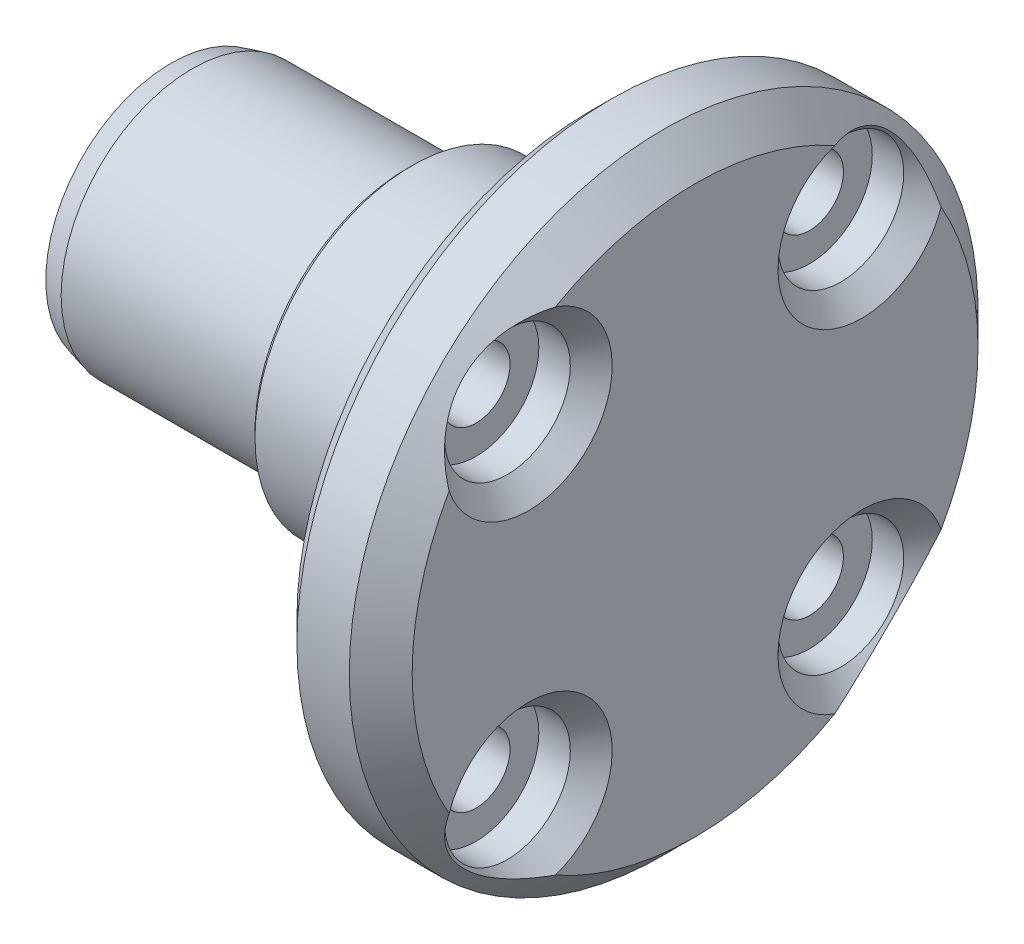
ISO-10303-21;
HEADER;
FILE_DESCRIPTION(('STEP AP214'),'2;1');
FILE_NAME('part.step','',(''),(''),'','','');
FILE_SCHEMA(('AUTOMOTIVE_DESIGN { 1 0 10303 214 1 1 1 1 }'));
ENDSEC;
DATA;
#1=APPLICATION_CONTEXT('core data for automotive mechanical design processes');
#2=APPLICATION_PROTOCOL_DEFINITION('international standard','automotive_design',2000,#1);
#3=PRODUCT_CONTEXT('',#1,'mechanical');
#4=PRODUCT('Part','Part','',(#3));
#5=PRODUCT_RELATED_PRODUCT_CATEGORY('part','',(#4));
#6=PRODUCT_DEFINITION_FORMATION('','',#4);
#7=PRODUCT_DEFINITION_CONTEXT('part definition',#1,'design');
#8=PRODUCT_DEFINITION('design','',#6,#7);
#9=PRODUCT_DEFINITION_SHAPE('','',#8);
#10=(LENGTH_UNIT() NAMED_UNIT(*) SI_UNIT(.MILLI.,.METRE.));
#11=(NAMED_UNIT(*) PLANE_ANGLE_UNIT() SI_UNIT($,.RADIAN.));
#12=(NAMED_UNIT(*) SI_UNIT($,.STERADIAN.) SOLID_ANGLE_UNIT());
#13=UNCERTAINTY_MEASURE_WITH_UNIT(LENGTH_MEASURE(1.E-05),#10,'distance_accuracy_value','');
#14=(GEOMETRIC_REPRESENTATION_CONTEXT(3) GLOBAL_UNCERTAINTY_ASSIGNED_CONTEXT((#13)) GLOBAL_UNIT_ASSIGNED_CONTEXT((#10,
#11,#12)) REPRESENTATION_CONTEXT('',''));
#15=CARTESIAN_POINT('',(0.,0.,0.));
#16=DIRECTION('',(0.,0.,1.));
#17=DIRECTION('',(1.,0.,0.));
#18=AXIS2_PLACEMENT_3D('',#15,#16,#17);
#19=CARTESIAN_POINT('',(0.,15.9099025766973,-15.9099025766973));
#20=DIRECTION('',(1.,0.,0.));
#21=DIRECTION('',(0.,0.,-1.));
#22=AXIS2_PLACEMENT_3D('',#19,#20,#21);
#23=CYLINDRICAL_SURFACE('',#22,3.25);
#24=CARTESIAN_POINT('',(40.,15.9099025766973,-15.9099025766973));
#25=DIRECTION('',(1.,0.,0.));
#26=DIRECTION('',(0.,0.,-1.));
#27=AXIS2_PLACEMENT_3D('',#24,#25,#26);
#28=CIRCLE('',#27,3.25);
#29=CARTESIAN_POINT('',(40.,15.9099025766973,-19.1599025766973));
#30=VERTEX_POINT('',#29);
#31=EDGE_CURVE('E154',#30,#30,#28,.T.);
#32=ORIENTED_EDGE('',*,*,#31,.F.);
#33=EDGE_LOOP('',(#32));
#34=FACE_BOUND('',#33,.T.);
#35=CARTESIAN_POINT('',(45.,15.9099025766973,-15.9099025766973));
#36=DIRECTION('',(1.,0.,0.));
#37=DIRECTION('',(0.,0.,-1.));
#38=AXIS2_PLACEMENT_3D('',#35,#36,#37);
#39=CIRCLE('',#38,3.25);
#40=CARTESIAN_POINT('',(45.,15.9099025766973,-19.1599025766973));
#41=VERTEX_POINT('',#40);
#42=EDGE_CURVE('E146',#41,#41,#39,.F.);
#43=ORIENTED_EDGE('',*,*,#42,.F.);
#44=EDGE_LOOP('',(#43));
#45=FACE_BOUND('',#44,.T.);
#46=ADVANCED_FACE('F43',(#34,#45),#23,.F.);
#47=CARTESIAN_POINT('',(0.,-15.9099025766973,-15.9099025766973));
#48=DIRECTION('',(1.,0.,0.));
#49=DIRECTION('',(0.,0.,-1.));
#50=AXIS2_PLACEMENT_3D('',#47,#48,#49);
#51=CYLINDRICAL_SURFACE('',#50,3.25);
#52=CARTESIAN_POINT('',(40.,-15.9099025766973,-15.9099025766973));
#53=DIRECTION('',(1.,0.,0.));
#54=DIRECTION('',(0.,0.,-1.));
#55=AXIS2_PLACEMENT_3D('',#52,#53,#54);
#56=CIRCLE('',#55,3.25);
#57=CARTESIAN_POINT('',(40.,-15.9099025766973,-19.1599025766973));
#58=VERTEX_POINT('',#57);
#59=EDGE_CURVE('E326',#58,#58,#56,.T.);
#60=ORIENTED_EDGE('',*,*,#59,.F.);
#61=EDGE_LOOP('',(#60));
#62=FACE_BOUND('',#61,.T.);
#63=CARTESIAN_POINT('',(45.,-15.9099025766973,-15.9099025766973));
#64=DIRECTION('',(1.,0.,0.));
#65=DIRECTION('',(0.,0.,-1.));
#66=AXIS2_PLACEMENT_3D('',#63,#64,#65);
#67=CIRCLE('',#66,3.25);
#68=CARTESIAN_POINT('',(45.,-15.9099025766973,-19.1599025766973));
#69=VERTEX_POINT('',#68);
#70=EDGE_CURVE('E147',#69,#69,#67,.F.);
#71=ORIENTED_EDGE('',*,*,#70,.F.);
#72=EDGE_LOOP('',(#71));
#73=FACE_BOUND('',#72,.T.);
#74=ADVANCED_FACE('F217',(#62,#73),#51,.F.);
#75=CARTESIAN_POINT('',(0.,-15.9099025766972,15.9099025766974));
#76=DIRECTION('',(1.,0.,0.));
#77=DIRECTION('',(0.,0.,-1.));
#78=AXIS2_PLACEMENT_3D('',#75,#76,#77);
#79=CYLINDRICAL_SURFACE('',#78,3.25);
#80=CARTESIAN_POINT('',(40.,-15.9099025766972,15.9099025766974));
#81=DIRECTION('',(1.,0.,0.));
#82=DIRECTION('',(0.,0.,-1.));
#83=AXIS2_PLACEMENT_3D('',#80,#81,#82);
#84=CIRCLE('',#83,3.25);
#85=CARTESIAN_POINT('',(40.,-15.9099025766972,12.6599025766974));
#86=VERTEX_POINT('',#85);
#87=EDGE_CURVE('E332',#86,#86,#84,.T.);
#88=ORIENTED_EDGE('',*,*,#87,.F.);
#89=EDGE_LOOP('',(#88));
#90=FACE_BOUND('',#89,.T.);
#91=CARTESIAN_POINT('',(45.,-15.9099025766972,15.9099025766974));
#92=DIRECTION('',(1.,0.,0.));
#93=DIRECTION('',(0.,0.,-1.));
#94=AXIS2_PLACEMENT_3D('',#91,#92,#93);
#95=CIRCLE('',#94,3.25);
#96=CARTESIAN_POINT('',(45.,-15.9099025766972,12.6599025766974));
#97=VERTEX_POINT('',#96);
#98=EDGE_CURVE('E145',#97,#97,#95,.F.);
#99=ORIENTED_EDGE('',*,*,#98,.F.);
#100=EDGE_LOOP('',(#99));
#101=FACE_BOUND('',#100,.T.);
#102=ADVANCED_FACE('F224',(#90,#101),#79,.F.);
#103=CARTESIAN_POINT('',(0.,15.9099025766975,15.9099025766972));
#104=DIRECTION('',(1.,0.,0.));
#105=DIRECTION('',(0.,0.,-1.));
#106=AXIS2_PLACEMENT_3D('',#103,#104,#105);
#107=CYLINDRICAL_SURFACE('',#106,3.25);
#108=CARTESIAN_POINT('',(40.,15.9099025766975,15.9099025766972));
#109=DIRECTION('',(1.,0.,0.));
#110=DIRECTION('',(0.,0.,-1.));
#111=AXIS2_PLACEMENT_3D('',#108,#109,#110);
#112=CIRCLE('',#111,3.25);
#113=CARTESIAN_POINT('',(40.,15.9099025766975,12.6599025766972));
#114=VERTEX_POINT('',#113);
#115=EDGE_CURVE('E337',#114,#114,#112,.T.);
#116=ORIENTED_EDGE('',*,*,#115,.F.);
#117=EDGE_LOOP('',(#116));
#118=FACE_BOUND('',#117,.T.);
#119=CARTESIAN_POINT('',(45.,15.9099025766975,15.9099025766972));
#120=DIRECTION('',(1.,0.,0.));
#121=DIRECTION('',(0.,0.,-1.));
#122=AXIS2_PLACEMENT_3D('',#119,#120,#121);
#123=CIRCLE('',#122,3.25);
#124=CARTESIAN_POINT('',(45.,15.9099025766975,12.6599025766972));
#125=VERTEX_POINT('',#124);
#126=EDGE_CURVE('E138',#125,#125,#123,.F.);
#127=ORIENTED_EDGE('',*,*,#126,.F.);
#128=EDGE_LOOP('',(#127));
#129=FACE_BOUND('',#128,.T.);
#130=ADVANCED_FACE('F235',(#118,#129),#107,.F.);
#131=CARTESIAN_POINT('',(0.,0.,0.));
#132=DIRECTION('',(1.,0.,0.));
#133=DIRECTION('',(0.,0.,-1.));
#134=AXIS2_PLACEMENT_3D('',#131,#132,#133);
#135=PLANE('',#134);
#136=CARTESIAN_POINT('',(0.,0.,0.));
#137=DIRECTION('',(1.,0.,0.));
#138=DIRECTION('',(0.,0.,-1.));
#139=AXIS2_PLACEMENT_3D('',#136,#137,#138);
#140=CIRCLE('',#139,11.9641016151378);
#141=CARTESIAN_POINT('',(0.,0.,-11.9641016151378));
#142=VERTEX_POINT('',#141);
#143=EDGE_CURVE('E287',#142,#142,#140,.F.);
#144=ORIENTED_EDGE('',*,*,#143,.T.);
#145=EDGE_LOOP('',(#144));
#146=FACE_BOUND('',#145,.T.);
#147=ADVANCED_FACE('F253',(#146),#135,.F.);
#148=CARTESIAN_POINT('',(-413.520497285991,0.,0.));
#149=DIRECTION('',(-1.,0.,0.));
#150=DIRECTION('',(0.,0.,1.));
#151=AXIS2_PLACEMENT_3D('',#148,#149,#150);
#152=CYLINDRICAL_SURFACE('',#151,12.5);
#153=CARTESIAN_POINT('',(21.5,0.,0.));
#154=DIRECTION('',(1.,0.,0.));
#155=DIRECTION('',(0.,0.,-1.));
#156=AXIS2_PLACEMENT_3D('',#153,#154,#155);
#157=CIRCLE('',#156,12.5);
#158=CARTESIAN_POINT('',(21.5,0.,-12.5));
#159=VERTEX_POINT('',#158);
#160=EDGE_CURVE('E134',#159,#159,#157,.F.);
#161=ORIENTED_EDGE('',*,*,#160,.T.);
#162=EDGE_LOOP('',(#161));
#163=FACE_BOUND('',#162,.T.);
#164=CARTESIAN_POINT('',(1.99999999999984,0.,0.));
#165=DIRECTION('',(1.,0.,0.));
#166=DIRECTION('',(0.,0.,-1.));
#167=AXIS2_PLACEMENT_3D('',#164,#165,#166);
#168=CIRCLE('',#167,12.5);
#169=CARTESIAN_POINT('',(1.99999999999984,0.,-12.5));
#170=VERTEX_POINT('',#169);
#171=EDGE_CURVE('E282',#170,#170,#168,.T.);
#172=ORIENTED_EDGE('',*,*,#171,.T.);
#173=EDGE_LOOP('',(#172));
#174=FACE_BOUND('',#173,.T.);
#175=ADVANCED_FACE('F252',(#163,#174),#152,.T.);
#176=CARTESIAN_POINT('',(22.5,12.5,0.));
#177=DIRECTION('',(1.,0.,0.));
#178=DIRECTION('',(0.,0.,-1.));
#179=AXIS2_PLACEMENT_3D('',#176,#177,#178);
#180=PLANE('',#179);
#181=CARTESIAN_POINT('',(22.5,0.,0.));
#182=DIRECTION('',(1.,0.,0.));
#183=DIRECTION('',(0.,0.,-1.));
#184=AXIS2_PLACEMENT_3D('',#181,#182,#183);
#185=CIRCLE('',#184,13.5);
#186=CARTESIAN_POINT('',(22.5,0.,-13.5));
#187=VERTEX_POINT('',#186);
#188=EDGE_CURVE('E131',#187,#187,#185,.T.);
#189=ORIENTED_EDGE('',*,*,#188,.T.);
#190=EDGE_LOOP('',(#189));
#191=FACE_BOUND('',#190,.T.);
#192=CARTESIAN_POINT('',(22.5,0.,0.));
#193=DIRECTION('',(1.,0.,0.));
#194=DIRECTION('',(0.,0.,-1.));
#195=AXIS2_PLACEMENT_3D('',#192,#193,#194);
#196=CIRCLE('',#195,14.5);
#197=CARTESIAN_POINT('',(22.5,0.,-14.5));
#198=VERTEX_POINT('',#197);
#199=EDGE_CURVE('E283',#198,#198,#196,.F.);
#200=ORIENTED_EDGE('',*,*,#199,.T.);
#201=EDGE_LOOP('',(#200));
#202=FACE_BOUND('',#201,.T.);
#203=ADVANCED_FACE('F250',(#191,#202),#180,.F.);
#204=CARTESIAN_POINT('',(-413.520497285991,0.,0.));
#205=DIRECTION('',(-1.,0.,0.));
#206=DIRECTION('',(0.,0.,1.));
#207=AXIS2_PLACEMENT_3D('',#204,#205,#206);
#208=CYLINDRICAL_SURFACE('',#207,15.);
#209=CARTESIAN_POINT('',(39.,0.,0.));
#210=DIRECTION('',(1.,0.,0.));
#211=DIRECTION('',(0.,0.,-1.));
#212=AXIS2_PLACEMENT_3D('',#209,#210,#211);
#213=CIRCLE('',#212,15.);
#214=CARTESIAN_POINT('',(39.,0.,-15.));
#215=VERTEX_POINT('',#214);
#216=EDGE_CURVE('E119',#215,#215,#213,.F.);
#217=ORIENTED_EDGE('',*,*,#216,.T.);
#218=EDGE_LOOP('',(#217));
#219=FACE_BOUND('',#218,.T.);
#220=CARTESIAN_POINT('',(23.,0.,0.));
#221=DIRECTION('',(1.,0.,0.));
#222=DIRECTION('',(0.,0.,-1.));
#223=AXIS2_PLACEMENT_3D('',#220,#221,#222);
#224=CIRCLE('',#223,15.);
#225=CARTESIAN_POINT('',(23.,0.,-15.));
#226=VERTEX_POINT('',#225);
#227=EDGE_CURVE('E279',#226,#226,#224,.T.);
#228=ORIENTED_EDGE('',*,*,#227,.T.);
#229=EDGE_LOOP('',(#228));
#230=FACE_BOUND('',#229,.T.);
#231=ADVANCED_FACE('F243',(#219,#230),#208,.T.);
#232=CARTESIAN_POINT('',(40.,15.,0.));
#233=DIRECTION('',(1.,0.,0.));
#234=DIRECTION('',(0.,0.,-1.));
#235=AXIS2_PLACEMENT_3D('',#232,#233,#234);
#236=PLANE('',#235);
#237=ORIENTED_EDGE('',*,*,#115,.T.);
#238=EDGE_LOOP('',(#237));
#239=FACE_BOUND('',#238,.T.);
#240=ORIENTED_EDGE('',*,*,#87,.T.);
#241=EDGE_LOOP('',(#240));
#242=FACE_BOUND('',#241,.T.);
#243=ORIENTED_EDGE('',*,*,#59,.T.);
#244=EDGE_LOOP('',(#243));
#245=FACE_BOUND('',#244,.T.);
#246=ORIENTED_EDGE('',*,*,#31,.T.);
#247=EDGE_LOOP('',(#246));
#248=FACE_BOUND('',#247,.T.);
#249=CARTESIAN_POINT('',(40.,0.,0.));
#250=DIRECTION('',(1.,0.,0.));
#251=DIRECTION('',(0.,0.,-1.));
#252=AXIS2_PLACEMENT_3D('',#249,#250,#251);
#253=CIRCLE('',#252,16.);
#254=CARTESIAN_POINT('',(40.,0.,-16.));
#255=VERTEX_POINT('',#254);
#256=EDGE_CURVE('E126',#255,#255,#253,.T.);
#257=ORIENTED_EDGE('',*,*,#256,.T.);
#258=EDGE_LOOP('',(#257));
#259=FACE_BOUND('',#258,.T.);
#260=CARTESIAN_POINT('',(40.,0.,0.));
#261=DIRECTION('',(1.,0.,0.));
#262=DIRECTION('',(0.,0.,-1.));
#263=AXIS2_PLACEMENT_3D('',#260,#261,#262);
#264=CIRCLE('',#263,28.);
#265=CARTESIAN_POINT('',(40.,0.,-28.));
#266=VERTEX_POINT('',#265);
#267=EDGE_CURVE('E281',#266,#266,#264,.F.);
#268=ORIENTED_EDGE('',*,*,#267,.T.);
#269=EDGE_LOOP('',(#268));
#270=FACE_BOUND('',#269,.T.);
#271=ADVANCED_FACE('F239',(#239,#242,#245,#248,#259,#270),#236,.F.);
#272=CARTESIAN_POINT('',(-413.520497285991,0.,0.));
#273=DIRECTION('',(-1.,0.,0.));
#274=DIRECTION('',(0.,0.,1.));
#275=AXIS2_PLACEMENT_3D('',#272,#273,#274);
#276=CYLINDRICAL_SURFACE('',#275,30.);
#277=CARTESIAN_POINT('',(47.,0.,0.));
#278=DIRECTION('',(-1.,0.,0.));
#279=DIRECTION('',(0.,0.,1.));
#280=AXIS2_PLACEMENT_3D('',#277,#278,#279);
#281=CIRCLE('',#280,30.);
#282=CARTESIAN_POINT('',(47.,0.,30.));
#283=VERTEX_POINT('',#282);
#284=EDGE_CURVE('E123',#283,#283,#281,.T.);
#285=ORIENTED_EDGE('',*,*,#284,.T.);
#286=EDGE_LOOP('',(#285));
#287=FACE_BOUND('',#286,.T.);
#288=CARTESIAN_POINT('',(42.,0.,0.));
#289=DIRECTION('',(1.,0.,0.));
#290=DIRECTION('',(0.,0.,-1.));
#291=AXIS2_PLACEMENT_3D('',#288,#289,#290);
#292=CIRCLE('',#291,30.);
#293=CARTESIAN_POINT('',(42.,0.,-30.));
#294=VERTEX_POINT('',#293);
#295=EDGE_CURVE('E291',#294,#294,#292,.T.);
#296=ORIENTED_EDGE('',*,*,#295,.T.);
#297=EDGE_LOOP('',(#296));
#298=FACE_BOUND('',#297,.T.);
#299=ADVANCED_FACE('F240',(#287,#298),#276,.T.);
#300=CARTESIAN_POINT('',(50.,30.,0.));
#301=DIRECTION('',(-1.,0.,0.));
#302=DIRECTION('',(0.,0.,1.));
#303=AXIS2_PLACEMENT_3D('',#300,#301,#302);
#304=PLANE('',#303);
#305=CARTESIAN_POINT('',(50.,0.,0.));
#306=DIRECTION('',(-1.,0.,0.));
#307=DIRECTION('',(0.,0.,1.));
#308=AXIS2_PLACEMENT_3D('',#305,#306,#307);
#309=CIRCLE('',#308,26.9999999999999);
#310=CARTESIAN_POINT('',(50.,13.3272740892091,23.4815622425573));
#311=VERTEX_POINT('',#310);
#312=CARTESIAN_POINT('',(50.,-13.3272740892072,23.4815622425584));
#313=VERTEX_POINT('',#312);
#314=EDGE_CURVE('E122',#311,#313,#309,.F.);
#315=ORIENTED_EDGE('',*,*,#314,.T.);
#316=CARTESIAN_POINT('',(50.,-15.9099025766972,15.9099025766975));
#317=DIRECTION('',(-1.,0.,0.));
#318=DIRECTION('',(0.,0.,1.));
#319=AXIS2_PLACEMENT_3D('',#316,#317,#318);
#320=CIRCLE('',#319,8.00000000000129);
#321=CARTESIAN_POINT('',(50.,-23.4815622425582,13.3272740892076));
#322=VERTEX_POINT('',#321);
#323=EDGE_CURVE('E157',#313,#322,#320,.T.);
#324=ORIENTED_EDGE('',*,*,#323,.T.);
#325=CARTESIAN_POINT('',(50.,-23.4815622425586,-13.3272740892067));
#326=VERTEX_POINT('',#325);
#327=EDGE_CURVE('E111',#322,#326,#309,.F.);
#328=ORIENTED_EDGE('',*,*,#327,.T.);
#329=CARTESIAN_POINT('',(50.,-15.9099025766975,-15.9099025766972));
#330=DIRECTION('',(-1.,0.,0.));
#331=DIRECTION('',(0.,0.,1.));
#332=AXIS2_PLACEMENT_3D('',#329,#330,#331);
#333=CIRCLE('',#332,8.00000000000167);
#334=CARTESIAN_POINT('',(50.,-13.3272740892071,-23.4815622425584));
#335=VERTEX_POINT('',#334);
#336=EDGE_CURVE('E94',#326,#335,#333,.T.);
#337=ORIENTED_EDGE('',*,*,#336,.T.);
#338=CARTESIAN_POINT('',(50.,13.3272740892082,-23.4815622425578));
#339=VERTEX_POINT('',#338);
#340=EDGE_CURVE('E108',#335,#339,#309,.F.);
#341=ORIENTED_EDGE('',*,*,#340,.T.);
#342=CARTESIAN_POINT('',(50.,15.9099025766972,-15.9099025766974));
#343=DIRECTION('',(-1.,0.,0.));
#344=DIRECTION('',(0.,0.,1.));
#345=AXIS2_PLACEMENT_3D('',#342,#343,#344);
#346=CIRCLE('',#345,8.00000000000041);
#347=CARTESIAN_POINT('',(50.,23.4815622425576,-13.3272740892086));
#348=VERTEX_POINT('',#347);
#349=EDGE_CURVE('E113',#339,#348,#346,.T.);
#350=ORIENTED_EDGE('',*,*,#349,.T.);
#351=CARTESIAN_POINT('',(50.,23.4815622425576,13.3272740892087));
#352=VERTEX_POINT('',#351);
#353=EDGE_CURVE('E117',#348,#352,#309,.F.);
#354=ORIENTED_EDGE('',*,*,#353,.T.);
#355=CARTESIAN_POINT('',(50.,15.9099025766975,15.9099025766972));
#356=DIRECTION('',(-1.,0.,0.));
#357=DIRECTION('',(0.,0.,1.));
#358=AXIS2_PLACEMENT_3D('',#355,#356,#357);
#359=CIRCLE('',#358,8.00000000000001);
#360=EDGE_CURVE('E115',#352,#311,#359,.T.);
#361=ORIENTED_EDGE('',*,*,#360,.T.);
#362=EDGE_LOOP('',(#315,#324,#328,#337,#341,#350,#354,#361));
#363=FACE_BOUND('',#362,.T.);
#364=ADVANCED_FACE('F106',(#363),#304,.F.);
#365=CARTESIAN_POINT('',(0.,0.,0.));
#366=DIRECTION('',(1.,0.,0.));
#367=DIRECTION('',(0.,0.,-1.));
#368=AXIS2_PLACEMENT_3D('',#365,#366,#367);
#369=CONICAL_SURFACE('',#368,11.9641016151378,0.261799387799145);
#370=ORIENTED_EDGE('',*,*,#171,.F.);
#371=EDGE_LOOP('',(#370));
#372=FACE_BOUND('',#371,.T.);
#373=ORIENTED_EDGE('',*,*,#143,.F.);
#374=EDGE_LOOP('',(#373));
#375=FACE_BOUND('',#374,.T.);
#376=ADVANCED_FACE('F236',(#372,#375),#369,.T.);
#377=CARTESIAN_POINT('',(22.5,0.,0.));
#378=DIRECTION('',(1.,0.,0.));
#379=DIRECTION('',(0.,0.,-1.));
#380=AXIS2_PLACEMENT_3D('',#377,#378,#379);
#381=CONICAL_SURFACE('',#380,14.5,0.785398163397459);
#382=ORIENTED_EDGE('',*,*,#227,.F.);
#383=EDGE_LOOP('',(#382));
#384=FACE_BOUND('',#383,.T.);
#385=ORIENTED_EDGE('',*,*,#199,.F.);
#386=EDGE_LOOP('',(#385));
#387=FACE_BOUND('',#386,.T.);
#388=ADVANCED_FACE('F261',(#384,#387),#381,.T.);
#389=CARTESIAN_POINT('',(40.,0.,0.));
#390=DIRECTION('',(1.,0.,0.));
#391=DIRECTION('',(0.,0.,-1.));
#392=AXIS2_PLACEMENT_3D('',#389,#390,#391);
#393=CONICAL_SURFACE('',#392,28.,0.785398163397449);
#394=ORIENTED_EDGE('',*,*,#295,.F.);
#395=EDGE_LOOP('',(#394));
#396=FACE_BOUND('',#395,.T.);
#397=ORIENTED_EDGE('',*,*,#267,.F.);
#398=EDGE_LOOP('',(#397));
#399=FACE_BOUND('',#398,.T.);
#400=ADVANCED_FACE('F179',(#396,#399),#393,.T.);
#401=CARTESIAN_POINT('',(47.,0.,0.));
#402=DIRECTION('',(-1.,0.,0.));
#403=DIRECTION('',(0.,0.,1.));
#404=AXIS2_PLACEMENT_3D('',#401,#402,#403);
#405=CONICAL_SURFACE('',#404,30.,0.785398163397453);
#406=ORIENTED_EDGE('',*,*,#327,.F.);
#407=CARTESIAN_POINT('',(50.,-23.4815622425582,13.3272740892076));
#408=CARTESIAN_POINT('',(49.8623244860714,-23.4501261029835,13.6615809085384));
#409=CARTESIAN_POINT('',(49.729847524722,-23.4060193855582,13.9971220723128));
#410=CARTESIAN_POINT('',(49.4770962688516,-23.2901308846266,14.6690349677443));
#411=CARTESIAN_POINT('',(49.3568557273336,-23.2182750397604,15.005406507941));
#412=CARTESIAN_POINT('',(49.130364607533,-23.044098697827,15.6778378924903));
#413=CARTESIAN_POINT('',(49.0242166728757,-22.9415706847337,16.0138794484197));
#414=CARTESIAN_POINT('',(48.8295157157687,-22.7044055048471,16.6793648815442));
#415=CARTESIAN_POINT('',(48.7409419766265,-22.569806560804,17.0088161103876));
#416=CARTESIAN_POINT('',(48.6077926268345,-22.3134344018236,17.5581018946699));
#417=CARTESIAN_POINT('',(48.5580366664604,-22.2002670031255,17.7807268217913));
#418=CARTESIAN_POINT('',(48.4690049388357,-21.9577334422976,18.2191201908146));
#419=CARTESIAN_POINT('',(48.4297264752503,-21.8283714603836,18.4348903841346));
#420=CARTESIAN_POINT('',(48.3624731952472,-21.5541150927226,18.857096419529));
#421=CARTESIAN_POINT('',(48.3344595512093,-21.409276276618,19.0635621083674));
#422=CARTESIAN_POINT('',(48.2900903846549,-21.1042659036492,19.4661796679442));
#423=CARTESIAN_POINT('',(48.2737347141895,-20.9440945413963,19.6623316695422));
#424=CARTESIAN_POINT('',(48.2529782152301,-20.6086471955302,20.0434409834205));
#425=CARTESIAN_POINT('',(48.2486285347439,-20.4333098597996,20.2283471279417));
#426=CARTESIAN_POINT('',(48.2521243327868,-20.0694228288624,20.5845437957797));
#427=CARTESIAN_POINT('',(48.2599699356902,-19.8808729989263,20.7558341802167));
#428=CARTESIAN_POINT('',(48.287695077658,-19.492041858547,21.0836731200354));
#429=CARTESIAN_POINT('',(48.307580891907,-19.2917544798609,21.2402139389581));
#430=CARTESIAN_POINT('',(48.3589796658958,-18.8812901088742,21.5376067757385));
#431=CARTESIAN_POINT('',(48.3904925605129,-18.6711131719704,21.6784588814622));
#432=CARTESIAN_POINT('',(48.4632222571038,-18.2502598824055,21.9393150015014));
#433=CARTESIAN_POINT('',(48.5040565993866,-18.0398638868651,22.0598800270941));
#434=CARTESIAN_POINT('',(48.5952975981466,-17.6131386639482,22.2858852932756));
#435=CARTESIAN_POINT('',(48.6457040569396,-17.3968095591817,22.3913258461373));
#436=CARTESIAN_POINT('',(48.7554740246399,-16.9591702576477,22.5874835389128));
#437=CARTESIAN_POINT('',(48.8148583395111,-16.7378495339623,22.6781654349596));
#438=CARTESIAN_POINT('',(48.9417252990491,-16.2920222701561,22.8448996268596));
#439=CARTESIAN_POINT('',(49.009209793041,-16.067515012884,22.9209485715568));
#440=CARTESIAN_POINT('',(49.1870466711792,-15.5038602181733,23.0933821941168));
#441=CARTESIAN_POINT('',(49.3019800268374,-15.1634383076975,23.1809636218455));
#442=CARTESIAN_POINT('',(49.5458457510178,-14.4814174201221,23.3265072868126));
#443=CARTESIAN_POINT('',(49.6747791170565,-14.1398183608304,23.3844674118187));
#444=CARTESIAN_POINT('',(49.9435868289789,-13.4601137155175,23.4728252608893));
#445=CARTESIAN_POINT('',(50.0833809907119,-13.1220001534713,23.5034073571108));
#446=CARTESIAN_POINT('',(50.3002689328816,-12.6175056752025,23.5307727053113));
#447=CARTESIAN_POINT('',(50.3736805300881,-12.4499677956794,23.5368133104263));
#448=CARTESIAN_POINT('',(50.5227811371483,-12.1157505422478,23.543025962824));
#449=CARTESIAN_POINT('',(50.5984706720326,-11.9490713767898,23.5431966466475));
#450=CARTESIAN_POINT('',(50.6752004593743,-11.7829063540803,23.5405647490687));
#451=B_SPLINE_CURVE_WITH_KNOTS('',3,(#407,#408,#409,#410,#411,#412,#413,#414,#415,#416,#417,
#418,#419,#420,#421,#422,#423,#424,#425,#426,#427,#428,#429,#430,#431,#432,#433,#434,#435,#436,
#437,#438,#439,#440,#441,#442,#443,#444,#445,#446,#447,#448,#449,#450),.UNSPECIFIED.,.F.,.F.,(4,
2,2,2,2,2,2,2,2,2,2,2,2,2,2,2,2,2,2,2,2,4),(0.,1.08886818828556,2.1806628363172,
3.28001794745952,4.37806932271815,5.14126897214217,5.90427202580824,6.66462213880451,
7.42496260218441,8.18853731054611,8.95211980631814,9.71610061326384,10.4800771412568,
11.2170440676808,11.953995775853,12.6926823009605,13.4315377950644,14.5392751691669,
15.6470915226554,16.7473901203332,17.296345280672,17.8454279508924),.UNSPECIFIED.);
#452=EDGE_CURVE('E187',#322,#313,#451,.T.);
#453=ORIENTED_EDGE('',*,*,#452,.T.);
#454=ORIENTED_EDGE('',*,*,#314,.F.);
#455=CARTESIAN_POINT('',(50.,13.3272740892091,23.4815622425573));
#456=CARTESIAN_POINT('',(49.8623244860714,13.6615809085398,23.4501261029826));
#457=CARTESIAN_POINT('',(49.729847524722,13.9971220723142,23.4060193855573));
#458=CARTESIAN_POINT('',(49.4770962688517,14.6690349677455,23.2901308846256));
#459=CARTESIAN_POINT('',(49.3568557273337,15.0054065079421,23.2182750397594));
#460=CARTESIAN_POINT('',(49.1303646075332,15.6778378924913,23.044098697826));
#461=CARTESIAN_POINT('',(49.024216672876,16.0138794484207,22.9415706847327));
#462=CARTESIAN_POINT('',(48.8295157157691,16.679364881545,22.7044055048461));
#463=CARTESIAN_POINT('',(48.7409419766269,17.0088161103883,22.5698065608029));
#464=CARTESIAN_POINT('',(48.607792626835,17.5581018946706,22.3134344018226));
#465=CARTESIAN_POINT('',(48.5580366664608,17.7807268217919,22.2002670031244));
#466=CARTESIAN_POINT('',(48.4690049388361,18.2191201908151,21.9577334422965));
#467=CARTESIAN_POINT('',(48.4297264752508,18.4348903841351,21.8283714603825));
#468=CARTESIAN_POINT('',(48.3624731952477,18.8570964195294,21.5541150927215));
#469=CARTESIAN_POINT('',(48.3344595512099,19.0635621083678,21.409276276617));
#470=CARTESIAN_POINT('',(48.2900903846555,19.4661796679446,21.1042659036481));
#471=CARTESIAN_POINT('',(48.2737347141901,19.6623316695424,20.9440945413952));
#472=CARTESIAN_POINT('',(48.2529782152308,20.0434409834207,20.6086471955291));
#473=CARTESIAN_POINT('',(48.2486285347445,20.2283471279419,20.4333098597985));
#474=CARTESIAN_POINT('',(48.2521243327875,20.5845437957798,20.0694228288614));
#475=CARTESIAN_POINT('',(48.2599699356909,20.7558341802168,19.8808729989252));
#476=CARTESIAN_POINT('',(48.2876950776587,21.0836731200354,19.4920418585461));
#477=CARTESIAN_POINT('',(48.3075808919077,21.240213938958,19.2917544798599));
#478=CARTESIAN_POINT('',(48.3589796658965,21.5376067757384,18.8812901088733));
#479=CARTESIAN_POINT('',(48.3904925605136,21.6784588814621,18.6711131719695));
#480=CARTESIAN_POINT('',(48.4632222571045,21.9393150015012,18.2502598824046));
#481=CARTESIAN_POINT('',(48.5040565993874,22.0598800270939,18.0398638868642));
#482=CARTESIAN_POINT('',(48.5952975981474,22.2858852932752,17.6131386639473));
#483=CARTESIAN_POINT('',(48.6457040569404,22.3913258461369,17.3968095591808));
#484=CARTESIAN_POINT('',(48.7554740246407,22.5874835389124,16.9591702576469));
#485=CARTESIAN_POINT('',(48.8148583395119,22.6781654349592,16.7378495339615));
#486=CARTESIAN_POINT('',(48.9417252990499,22.8448996268592,16.2920222701554));
#487=CARTESIAN_POINT('',(49.0092097930418,22.9209485715563,16.0675150128832));
#488=CARTESIAN_POINT('',(49.18704667118,23.0933821941163,15.5038602181725));
#489=CARTESIAN_POINT('',(49.3019800268382,23.180963621845,15.1634383076968));
#490=CARTESIAN_POINT('',(49.5458457510187,23.326507286812,14.4814174201214));
#491=CARTESIAN_POINT('',(49.6747791170574,23.3844674118181,14.1398183608297));
#492=CARTESIAN_POINT('',(49.9435868289798,23.4728252608887,13.4601137155168));
#493=CARTESIAN_POINT('',(50.0833809907128,23.5034073571102,13.1220001534706));
#494=CARTESIAN_POINT('',(50.3002689328825,23.5307727053106,12.6175056752018));
#495=CARTESIAN_POINT('',(50.3736805300891,23.5368133104256,12.4499677956787));
#496=CARTESIAN_POINT('',(50.5227811371492,23.5430259628233,12.1157505422471));
#497=CARTESIAN_POINT('',(50.5984706720335,23.5431966466467,11.9490713767891));
#498=CARTESIAN_POINT('',(50.6752004593753,23.540564749068,11.7829063540797));
#499=B_SPLINE_CURVE_WITH_KNOTS('',3,(#455,#456,#457,#458,#459,#460,#461,#462,#463,#464,#465,
#466,#467,#468,#469,#470,#471,#472,#473,#474,#475,#476,#477,#478,#479,#480,#481,#482,#483,#484,
#485,#486,#487,#488,#489,#490,#491,#492,#493,#494,#495,#496,#497,#498),.UNSPECIFIED.,.F.,.F.,(4,
2,2,2,2,2,2,2,2,2,2,2,2,2,2,2,2,2,2,2,2,4),(0.,1.08886818828535,2.18066283631678,
3.2800179474589,4.37806932271732,5.14126897214124,5.90427202580722,6.6646221388034,
7.42496260218319,8.18853731054479,8.95211980631673,9.71610061326232,10.4800771412552,
11.2170440676791,11.9539957758512,12.6926823009587,13.4315377950625,14.539275169165,
15.6470915226536,16.7473901203313,17.2963452806701,17.8454279508905),.UNSPECIFIED.);
#500=EDGE_CURVE('E99',#311,#352,#499,.T.);
#501=ORIENTED_EDGE('',*,*,#500,.T.);
#502=ORIENTED_EDGE('',*,*,#353,.F.);
#503=CARTESIAN_POINT('',(50.,23.4815622425576,-13.3272740892086));
#504=CARTESIAN_POINT('',(49.8623244860714,23.4501261029829,-13.6615809085393));
#505=CARTESIAN_POINT('',(49.729847524722,23.4060193855576,-13.9971220723138));
#506=CARTESIAN_POINT('',(49.4770962688517,23.2901308846259,-14.6690349677451));
#507=CARTESIAN_POINT('',(49.3568557273337,23.2182750397597,-15.0054065079418));
#508=CARTESIAN_POINT('',(49.1303646075331,23.0440986978263,-15.677837892491));
#509=CARTESIAN_POINT('',(49.0242166728759,22.941570684733,-16.0138794484204));
#510=CARTESIAN_POINT('',(48.829515715769,22.7044055048464,-16.6793648815447));
#511=CARTESIAN_POINT('',(48.7409419766268,22.5698065608033,-17.0088161103881));
#512=CARTESIAN_POINT('',(48.6077926268348,22.3134344018229,-17.5581018946704));
#513=CARTESIAN_POINT('',(48.5580366664607,22.2002670031248,-17.7807268217917));
#514=CARTESIAN_POINT('',(48.469004938836,21.9577334422969,-18.2191201908149));
#515=CARTESIAN_POINT('',(48.4297264752506,21.8283714603829,-18.434890384135));
#516=CARTESIAN_POINT('',(48.3624731952476,21.5541150927219,-18.8570964195293));
#517=CARTESIAN_POINT('',(48.3344595512097,21.4092762766173,-19.0635621083677));
#518=CARTESIAN_POINT('',(48.2900903846553,21.1042659036484,-19.4661796679444));
#519=CARTESIAN_POINT('',(48.2737347141899,20.9440945413955,-19.6623316695424));
#520=CARTESIAN_POINT('',(48.2529782152306,20.6086471955295,-20.0434409834206));
#521=CARTESIAN_POINT('',(48.2486285347443,20.4333098597989,-20.2283471279418));
#522=CARTESIAN_POINT('',(48.2521243327873,20.0694228288617,-20.5845437957798));
#523=CARTESIAN_POINT('',(48.2599699356907,19.8808729989256,-20.7558341802167));
#524=CARTESIAN_POINT('',(48.2876950776585,19.4920418585464,-21.0836731200354));
#525=CARTESIAN_POINT('',(48.3075808919075,19.2917544798602,-21.2402139389581));
#526=CARTESIAN_POINT('',(48.3589796658963,18.8812901088736,-21.5376067757384));
#527=CARTESIAN_POINT('',(48.3904925605134,18.6711131719698,-21.6784588814621));
#528=CARTESIAN_POINT('',(48.4632222571043,18.2502598824049,-21.9393150015012));
#529=CARTESIAN_POINT('',(48.5040565993871,18.0398638868645,-22.059880027094));
#530=CARTESIAN_POINT('',(48.5952975981471,17.6131386639476,-22.2858852932753));
#531=CARTESIAN_POINT('',(48.6457040569401,17.3968095591811,-22.391325846137));
#532=CARTESIAN_POINT('',(48.7554740246405,16.9591702576472,-22.5874835389126));
#533=CARTESIAN_POINT('',(48.8148583395116,16.7378495339618,-22.6781654349593));
#534=CARTESIAN_POINT('',(48.9417252990497,16.2920222701556,-22.8448996268593));
#535=CARTESIAN_POINT('',(49.0092097930415,16.0675150128835,-22.9209485715565));
#536=CARTESIAN_POINT('',(49.1870466711798,15.5038602181728,-23.0933821941164));
#537=CARTESIAN_POINT('',(49.301980026838,15.1634383076971,-23.1809636218451));
#538=CARTESIAN_POINT('',(49.5458457510184,14.4814174201216,-23.3265072868122));
#539=CARTESIAN_POINT('',(49.6747791170571,14.1398183608299,-23.3844674118183));
#540=CARTESIAN_POINT('',(49.9435868289796,13.460113715517,-23.4728252608888));
#541=CARTESIAN_POINT('',(50.0833809907125,13.1220001534708,-23.5034073571104));
#542=CARTESIAN_POINT('',(50.3002689328822,12.617505675202,-23.5307727053108));
#543=CARTESIAN_POINT('',(50.3736805300888,12.4499677956789,-23.5368133104258));
#544=CARTESIAN_POINT('',(50.5227811371489,12.1157505422473,-23.5430259628235));
#545=CARTESIAN_POINT('',(50.5984706720332,11.9490713767894,-23.543196646647));
#546=CARTESIAN_POINT('',(50.675200459375,11.7829063540799,-23.5405647490682));
#547=B_SPLINE_CURVE_WITH_KNOTS('',3,(#503,#504,#505,#506,#507,#508,#509,#510,#511,#512,#513,
#514,#515,#516,#517,#518,#519,#520,#521,#522,#523,#524,#525,#526,#527,#528,#529,#530,#531,#532,
#533,#534,#535,#536,#537,#538,#539,#540,#541,#542,#543,#544,#545,#546),.UNSPECIFIED.,.F.,.F.,(4,
2,2,2,2,2,2,2,2,2,2,2,2,2,2,2,2,2,2,2,2,4),(0.,1.08886818828541,2.18066283631691,
3.28001794745909,4.37806932271758,5.14126897214153,5.90427202580754,6.66462213880375,
7.42496260218357,8.1885373105452,8.95211980631717,9.71610061326279,10.4800771412557,
11.2170440676796,11.9539957758518,12.6926823009593,13.4315377950631,14.5392751691656,
15.6470915226541,16.7473901203318,17.2963452806707,17.8454279508911),.UNSPECIFIED.);
#548=EDGE_CURVE('E103',#348,#339,#547,.T.);
#549=ORIENTED_EDGE('',*,*,#548,.T.);
#550=ORIENTED_EDGE('',*,*,#340,.F.);
#551=CARTESIAN_POINT('',(50.,-13.3272740892071,-23.4815622425584));
#552=CARTESIAN_POINT('',(49.8623244860714,-13.6615809085379,-23.4501261029838));
#553=CARTESIAN_POINT('',(49.7298475247219,-13.9971220723124,-23.4060193855585));
#554=CARTESIAN_POINT('',(49.4770962688516,-14.6690349677439,-23.2901308846269));
#555=CARTESIAN_POINT('',(49.3568557273335,-15.0054065079406,-23.2182750397607));
#556=CARTESIAN_POINT('',(49.1303646075329,-15.67783789249,-23.0440986978272));
#557=CARTESIAN_POINT('',(49.0242166728756,-16.0138794484195,-22.941570684734));
#558=CARTESIAN_POINT('',(48.8295157157686,-16.6793648815439,-22.7044055048474));
#559=CARTESIAN_POINT('',(48.7409419766264,-17.0088161103874,-22.5698065608043));
#560=CARTESIAN_POINT('',(48.6077926268344,-17.5581018946698,-22.3134344018239));
#561=CARTESIAN_POINT('',(48.5580366664603,-17.7807268217911,-22.2002670031258));
#562=CARTESIAN_POINT('',(48.4690049388355,-18.2191201908144,-21.9577334422979));
#563=CARTESIAN_POINT('',(48.4297264752501,-18.4348903841345,-21.8283714603839));
#564=CARTESIAN_POINT('',(48.3624731952471,-18.8570964195289,-21.5541150927229));
#565=CARTESIAN_POINT('',(48.3344595512092,-19.0635621083673,-21.4092762766184));
#566=CARTESIAN_POINT('',(48.2900903846548,-19.4661796679442,-21.1042659036495));
#567=CARTESIAN_POINT('',(48.2737347141893,-19.6623316695421,-20.9440945413966));
#568=CARTESIAN_POINT('',(48.25297821523,-20.0434409834204,-20.6086471955305));
#569=CARTESIAN_POINT('',(48.2486285347437,-20.2283471279417,-20.4333098597999));
#570=CARTESIAN_POINT('',(48.2521243327866,-20.5845437957797,-20.0694228288627));
#571=CARTESIAN_POINT('',(48.25996993569,-20.7558341802167,-19.8808729989266));
#572=CARTESIAN_POINT('',(48.2876950776578,-21.0836731200355,-19.4920418585473));
#573=CARTESIAN_POINT('',(48.3075808919068,-21.2402139389581,-19.2917544798612));
#574=CARTESIAN_POINT('',(48.3589796658956,-21.5376067757386,-18.8812901088745));
#575=CARTESIAN_POINT('',(48.3904925605126,-21.6784588814623,-18.6711131719707));
#576=CARTESIAN_POINT('',(48.4632222571035,-21.9393150015014,-18.2502598824057));
#577=CARTESIAN_POINT('',(48.5040565993864,-22.0598800270942,-18.0398638868654));
#578=CARTESIAN_POINT('',(48.5952975981464,-22.2858852932756,-17.6131386639485));
#579=CARTESIAN_POINT('',(48.6457040569393,-22.3913258461373,-17.3968095591819));
#580=CARTESIAN_POINT('',(48.7554740246397,-22.5874835389129,-16.959170257648));
#581=CARTESIAN_POINT('',(48.8148583395108,-22.6781654349597,-16.7378495339626));
#582=CARTESIAN_POINT('',(48.9417252990489,-22.8448996268597,-16.2920222701564));
#583=CARTESIAN_POINT('',(49.0092097930407,-22.9209485715569,-16.0675150128842));
#584=CARTESIAN_POINT('',(49.1870466711789,-23.0933821941169,-15.5038602181735));
#585=CARTESIAN_POINT('',(49.3019800268371,-23.1809636218456,-15.1634383076978));
#586=CARTESIAN_POINT('',(49.5458457510175,-23.3265072868128,-14.4814174201223));
#587=CARTESIAN_POINT('',(49.6747791170562,-23.3844674118189,-14.1398183608306));
#588=CARTESIAN_POINT('',(49.9435868289787,-23.4728252608895,-13.4601137155177));
#589=CARTESIAN_POINT('',(50.0833809907116,-23.503407357111,-13.1220001534715));
#590=CARTESIAN_POINT('',(50.3002689328813,-23.5307727053115,-12.6175056752027));
#591=CARTESIAN_POINT('',(50.3736805300878,-23.5368133104265,-12.4499677956796));
#592=CARTESIAN_POINT('',(50.522781137148,-23.5430259628243,-12.115750542248));
#593=CARTESIAN_POINT('',(50.5984706720323,-23.5431966466477,-11.94907137679));
#594=CARTESIAN_POINT('',(50.675200459374,-23.5405647490689,-11.7829063540806));
#595=B_SPLINE_CURVE_WITH_KNOTS('',3,(#551,#552,#553,#554,#555,#556,#557,#558,#559,#560,#561,
#562,#563,#564,#565,#566,#567,#568,#569,#570,#571,#572,#573,#574,#575,#576,#577,#578,#579,#580,
#581,#582,#583,#584,#585,#586,#587,#588,#589,#590,#591,#592,#593,#594),.UNSPECIFIED.,.F.,.F.,(4,
2,2,2,2,2,2,2,2,2,2,2,2,2,2,2,2,2,2,2,2,4),(0.,1.08886818828561,2.18066283631731,
3.2800179474597,4.37806932271839,5.14126897214243,5.90427202580853,6.66462213880483,
7.42496260218475,8.18853731054647,8.95211980631854,9.71610061326426,10.4800771412572,
11.2170440676813,11.9539957758535,12.692682300961,13.4315377950649,14.5392751691674,
15.647091522656,16.7473901203337,17.2963452806726,17.8454279508929),.UNSPECIFIED.);
#596=EDGE_CURVE('E95',#335,#326,#595,.T.);
#597=ORIENTED_EDGE('',*,*,#596,.T.);
#598=EDGE_LOOP('',(#406,#453,#454,#501,#502,#549,#550,#597));
#599=FACE_BOUND('',#598,.T.);
#600=ORIENTED_EDGE('',*,*,#284,.F.);
#601=EDGE_LOOP('',(#600));
#602=FACE_BOUND('',#601,.T.);
#603=ADVANCED_FACE('F114',(#599,#602),#405,.T.);
#604=CARTESIAN_POINT('',(39.,0.,0.));
#605=DIRECTION('',(1.,0.,0.));
#606=DIRECTION('',(0.,0.,-1.));
#607=AXIS2_PLACEMENT_3D('',#604,#605,#606);
#608=TOROIDAL_SURFACE('',#607,16.,1.);
#609=ORIENTED_EDGE('',*,*,#256,.F.);
#610=EDGE_LOOP('',(#609));
#611=FACE_BOUND('',#610,.T.);
#612=ORIENTED_EDGE('',*,*,#216,.F.);
#613=EDGE_LOOP('',(#612));
#614=FACE_BOUND('',#613,.T.);
#615=ADVANCED_FACE('F177',(#611,#614),#608,.F.);
#616=CARTESIAN_POINT('',(21.5,0.,0.));
#617=DIRECTION('',(1.,0.,0.));
#618=DIRECTION('',(0.,0.,-1.));
#619=AXIS2_PLACEMENT_3D('',#616,#617,#618);
#620=TOROIDAL_SURFACE('',#619,13.5,1.);
#621=ORIENTED_EDGE('',*,*,#188,.F.);
#622=EDGE_LOOP('',(#621));
#623=FACE_BOUND('',#622,.T.);
#624=ORIENTED_EDGE('',*,*,#160,.F.);
#625=EDGE_LOOP('',(#624));
#626=FACE_BOUND('',#625,.T.);
#627=ADVANCED_FACE('F351',(#623,#626),#620,.F.);
#628=CARTESIAN_POINT('',(45.,15.9099025766975,15.9099025766972));
#629=DIRECTION('',(1.,0.,0.));
#630=DIRECTION('',(0.,0.,-1.));
#631=AXIS2_PLACEMENT_3D('',#628,#629,#630);
#632=PLANE('',#631);
#633=CARTESIAN_POINT('',(45.,15.9099025766975,15.9099025766972));
#634=DIRECTION('',(1.,0.,0.));
#635=DIRECTION('',(0.,0.,-1.));
#636=AXIS2_PLACEMENT_3D('',#633,#634,#635);
#637=CIRCLE('',#636,6.);
#638=CARTESIAN_POINT('',(45.,15.9099025766975,9.90990257669718));
#639=VERTEX_POINT('',#638);
#640=EDGE_CURVE('E141',#639,#639,#637,.T.);
#641=ORIENTED_EDGE('',*,*,#640,.T.);
#642=EDGE_LOOP('',(#641));
#643=FACE_BOUND('',#642,.T.);
#644=ORIENTED_EDGE('',*,*,#126,.T.);
#645=EDGE_LOOP('',(#644));
#646=FACE_BOUND('',#645,.T.);
#647=ADVANCED_FACE('F347',(#643,#646),#632,.T.);
#648=CARTESIAN_POINT('',(45.,15.9099025766975,15.9099025766972));
#649=DIRECTION('',(1.,0.,0.));
#650=DIRECTION('',(0.,0.,-1.));
#651=AXIS2_PLACEMENT_3D('',#648,#649,#650);
#652=CYLINDRICAL_SURFACE('',#651,6.);
#653=CARTESIAN_POINT('',(48.,15.9099025766975,15.9099025766972));
#654=DIRECTION('',(-1.,0.,0.));
#655=DIRECTION('',(0.,0.,1.));
#656=AXIS2_PLACEMENT_3D('',#653,#654,#655);
#657=CIRCLE('',#656,6.);
#658=CARTESIAN_POINT('',(48.,13.9729312110812,21.5886473260923));
#659=VERTEX_POINT('',#658);
#660=EDGE_CURVE('E302',#659,#659,#657,.F.);
#661=ORIENTED_EDGE('',*,*,#660,.T.);
#662=EDGE_LOOP('',(#661));
#663=FACE_BOUND('',#662,.T.);
#664=ORIENTED_EDGE('',*,*,#640,.F.);
#665=EDGE_LOOP('',(#664));
#666=FACE_BOUND('',#665,.T.);
#667=ADVANCED_FACE('F346',(#663,#666),#652,.F.);
#668=CARTESIAN_POINT('',(45.,-15.9099025766972,15.9099025766975));
#669=DIRECTION('',(1.,0.,0.));
#670=DIRECTION('',(0.,0.,-1.));
#671=AXIS2_PLACEMENT_3D('',#668,#669,#670);
#672=PLANE('',#671);
#673=CARTESIAN_POINT('',(45.,-15.9099025766972,15.9099025766975));
#674=DIRECTION('',(1.,0.,0.));
#675=DIRECTION('',(0.,0.,-1.));
#676=AXIS2_PLACEMENT_3D('',#673,#674,#675);
#677=CIRCLE('',#676,6.00000000000128);
#678=CARTESIAN_POINT('',(45.,-15.9099025766972,9.90990257669617));
#679=VERTEX_POINT('',#678);
#680=EDGE_CURVE('E319',#679,#679,#677,.T.);
#681=ORIENTED_EDGE('',*,*,#680,.T.);
#682=EDGE_LOOP('',(#681));
#683=FACE_BOUND('',#682,.T.);
#684=ORIENTED_EDGE('',*,*,#98,.T.);
#685=EDGE_LOOP('',(#684));
#686=FACE_BOUND('',#685,.T.);
#687=ADVANCED_FACE('F356',(#683,#686),#672,.T.);
#688=CARTESIAN_POINT('',(45.,-15.9099025766972,15.9099025766975));
#689=DIRECTION('',(1.,0.,0.));
#690=DIRECTION('',(0.,0.,-1.));
#691=AXIS2_PLACEMENT_3D('',#688,#689,#690);
#692=CYLINDRICAL_SURFACE('',#691,6.00000000000128);
#693=CARTESIAN_POINT('',(48.,-15.9099025766972,15.9099025766975));
#694=DIRECTION('',(-1.,0.,0.));
#695=DIRECTION('',(0.,0.,1.));
#696=AXIS2_PLACEMENT_3D('',#693,#694,#695);
#697=CIRCLE('',#696,6.00000000000128);
#698=CARTESIAN_POINT('',(48.,-21.5886473260932,13.9729312110799));
#699=VERTEX_POINT('',#698);
#700=EDGE_CURVE('E137',#699,#699,#697,.F.);
#701=ORIENTED_EDGE('',*,*,#700,.T.);
#702=EDGE_LOOP('',(#701));
#703=FACE_BOUND('',#702,.T.);
#704=ORIENTED_EDGE('',*,*,#680,.F.);
#705=EDGE_LOOP('',(#704));
#706=FACE_BOUND('',#705,.T.);
#707=ADVANCED_FACE('F375',(#703,#706),#692,.F.);
#708=CARTESIAN_POINT('',(45.,-15.9099025766975,-15.9099025766972));
#709=DIRECTION('',(1.,0.,0.));
#710=DIRECTION('',(0.,0.,-1.));
#711=AXIS2_PLACEMENT_3D('',#708,#709,#710);
#712=PLANE('',#711);
#713=CARTESIAN_POINT('',(45.,-15.9099025766975,-15.9099025766972));
#714=DIRECTION('',(1.,0.,0.));
#715=DIRECTION('',(0.,0.,-1.));
#716=AXIS2_PLACEMENT_3D('',#713,#714,#715);
#717=CIRCLE('',#716,6.00000000000168);
#718=CARTESIAN_POINT('',(45.,-15.9099025766975,-21.9099025766989));
#719=VERTEX_POINT('',#718);
#720=EDGE_CURVE('E317',#719,#719,#717,.T.);
#721=ORIENTED_EDGE('',*,*,#720,.T.);
#722=EDGE_LOOP('',(#721));
#723=FACE_BOUND('',#722,.T.);
#724=ORIENTED_EDGE('',*,*,#70,.T.);
#725=EDGE_LOOP('',(#724));
#726=FACE_BOUND('',#725,.T.);
#727=ADVANCED_FACE('F315',(#723,#726),#712,.T.);
#728=CARTESIAN_POINT('',(45.,-15.9099025766975,-15.9099025766972));
#729=DIRECTION('',(1.,0.,0.));
#730=DIRECTION('',(0.,0.,-1.));
#731=AXIS2_PLACEMENT_3D('',#728,#729,#730);
#732=CYLINDRICAL_SURFACE('',#731,6.00000000000168);
#733=CARTESIAN_POINT('',(48.,-15.9099025766975,-15.9099025766972));
#734=DIRECTION('',(-1.,0.,0.));
#735=DIRECTION('',(0.,0.,1.));
#736=AXIS2_PLACEMENT_3D('',#733,#734,#735);
#737=CIRCLE('',#736,6.00000000000168);
#738=CARTESIAN_POINT('',(48.,-13.9729312110796,-21.5886473260935));
#739=VERTEX_POINT('',#738);
#740=EDGE_CURVE('E52',#739,#739,#737,.F.);
#741=ORIENTED_EDGE('',*,*,#740,.T.);
#742=EDGE_LOOP('',(#741));
#743=FACE_BOUND('',#742,.T.);
#744=ORIENTED_EDGE('',*,*,#720,.F.);
#745=EDGE_LOOP('',(#744));
#746=FACE_BOUND('',#745,.T.);
#747=ADVANCED_FACE('F308',(#743,#746),#732,.F.);
#748=CARTESIAN_POINT('',(45.,15.9099025766972,-15.9099025766974));
#749=DIRECTION('',(1.,0.,0.));
#750=DIRECTION('',(0.,0.,-1.));
#751=AXIS2_PLACEMENT_3D('',#748,#749,#750);
#752=PLANE('',#751);
#753=CARTESIAN_POINT('',(45.,15.9099025766972,-15.9099025766974));
#754=DIRECTION('',(1.,0.,0.));
#755=DIRECTION('',(0.,0.,-1.));
#756=AXIS2_PLACEMENT_3D('',#753,#754,#755);
#757=CIRCLE('',#756,6.00000000000039);
#758=CARTESIAN_POINT('',(45.,15.9099025766972,-21.9099025766978));
#759=VERTEX_POINT('',#758);
#760=EDGE_CURVE('E316',#759,#759,#757,.T.);
#761=ORIENTED_EDGE('',*,*,#760,.T.);
#762=EDGE_LOOP('',(#761));
#763=FACE_BOUND('',#762,.T.);
#764=ORIENTED_EDGE('',*,*,#42,.T.);
#765=EDGE_LOOP('',(#764));
#766=FACE_BOUND('',#765,.T.);
#767=ADVANCED_FACE('F311',(#763,#766),#752,.T.);
#768=CARTESIAN_POINT('',(45.,15.9099025766972,-15.9099025766974));
#769=DIRECTION('',(1.,0.,0.));
#770=DIRECTION('',(0.,0.,-1.));
#771=AXIS2_PLACEMENT_3D('',#768,#769,#770);
#772=CYLINDRICAL_SURFACE('',#771,6.00000000000039);
#773=CARTESIAN_POINT('',(48.,15.9099025766972,-15.9099025766974));
#774=DIRECTION('',(-1.,0.,0.));
#775=DIRECTION('',(0.,0.,1.));
#776=AXIS2_PLACEMENT_3D('',#773,#774,#775);
#777=CIRCLE('',#776,6.00000000000039);
#778=CARTESIAN_POINT('',(48.,21.5886473260926,-13.9729312110808));
#779=VERTEX_POINT('',#778);
#780=EDGE_CURVE('E11',#779,#779,#777,.F.);
#781=ORIENTED_EDGE('',*,*,#780,.T.);
#782=EDGE_LOOP('',(#781));
#783=FACE_BOUND('',#782,.T.);
#784=ORIENTED_EDGE('',*,*,#760,.F.);
#785=EDGE_LOOP('',(#784));
#786=FACE_BOUND('',#785,.T.);
#787=ADVANCED_FACE('F385',(#783,#786),#772,.F.);
#788=CARTESIAN_POINT('',(48.,-15.9099025766972,15.9099025766975));
#789=DIRECTION('',(1.,0.,0.));
#790=DIRECTION('',(0.,0.,-1.));
#791=AXIS2_PLACEMENT_3D('',#788,#789,#790);
#792=CONICAL_SURFACE('',#791,6.00000000000128,0.785398163397452);
#793=ORIENTED_EDGE('',*,*,#452,.F.);
#794=ORIENTED_EDGE('',*,*,#323,.F.);
#795=EDGE_LOOP('',(#793,#794));
#796=FACE_BOUND('',#795,.T.);
#797=ORIENTED_EDGE('',*,*,#700,.F.);
#798=EDGE_LOOP('',(#797));
#799=FACE_BOUND('',#798,.T.);
#800=ADVANCED_FACE('F207',(#796,#799),#792,.F.);
#801=CARTESIAN_POINT('',(48.,15.9099025766975,15.9099025766972));
#802=DIRECTION('',(1.,0.,0.));
#803=DIRECTION('',(0.,0.,-1.));
#804=AXIS2_PLACEMENT_3D('',#801,#802,#803);
#805=CONICAL_SURFACE('',#804,6.,0.785398163397449);
#806=ORIENTED_EDGE('',*,*,#500,.F.);
#807=ORIENTED_EDGE('',*,*,#360,.F.);
#808=EDGE_LOOP('',(#806,#807));
#809=FACE_BOUND('',#808,.T.);
#810=ORIENTED_EDGE('',*,*,#660,.F.);
#811=EDGE_LOOP('',(#810));
#812=FACE_BOUND('',#811,.T.);
#813=ADVANCED_FACE('F196',(#809,#812),#805,.F.);
#814=CARTESIAN_POINT('',(48.,-15.9099025766975,-15.9099025766972));
#815=DIRECTION('',(1.,0.,0.));
#816=DIRECTION('',(0.,0.,-1.));
#817=AXIS2_PLACEMENT_3D('',#814,#815,#816);
#818=CONICAL_SURFACE('',#817,6.00000000000168,0.785398163397451);
#819=ORIENTED_EDGE('',*,*,#596,.F.);
#820=ORIENTED_EDGE('',*,*,#336,.F.);
#821=EDGE_LOOP('',(#819,#820));
#822=FACE_BOUND('',#821,.T.);
#823=ORIENTED_EDGE('',*,*,#740,.F.);
#824=EDGE_LOOP('',(#823));
#825=FACE_BOUND('',#824,.T.);
#826=ADVANCED_FACE('F93',(#822,#825),#818,.F.);
#827=CARTESIAN_POINT('',(48.,15.9099025766972,-15.9099025766974));
#828=DIRECTION('',(1.,0.,0.));
#829=DIRECTION('',(0.,0.,-1.));
#830=AXIS2_PLACEMENT_3D('',#827,#828,#829);
#831=CONICAL_SURFACE('',#830,6.00000000000039,0.78539816339745);
#832=ORIENTED_EDGE('',*,*,#548,.F.);
#833=ORIENTED_EDGE('',*,*,#349,.F.);
#834=EDGE_LOOP('',(#832,#833));
#835=FACE_BOUND('',#834,.T.);
#836=ORIENTED_EDGE('',*,*,#780,.F.);
#837=EDGE_LOOP('',(#836));
#838=FACE_BOUND('',#837,.T.);
#839=ADVANCED_FACE('F46',(#835,#838),#831,.F.);
#840=CLOSED_SHELL('',(#46,#74,#102,#130,#147,#175,#203,#231,#271,#299,#364,#376,#388,#400,#603,
#615,#627,#647,#667,#687,#707,#727,#747,#767,#787,#800,#813,#826,#839));
#841=MANIFOLD_SOLID_BREP('B2',#840);
#842=ADVANCED_BREP_SHAPE_REPRESENTATION('',(#18,#841),#14);
#843=SHAPE_DEFINITION_REPRESENTATION(#9,#842);
ENDSEC;
END-ISO-10303-21;
